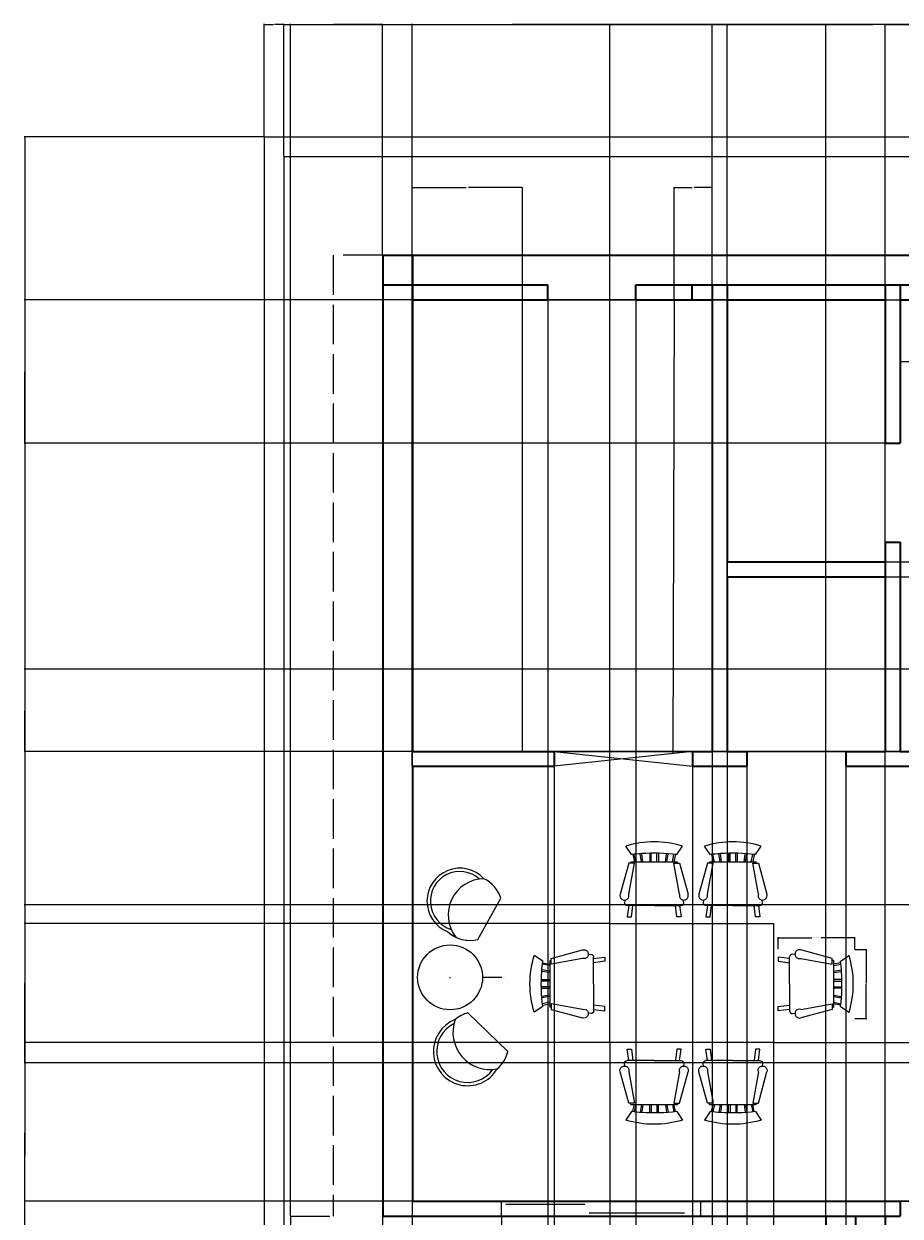
# Model space of a CAD drawing. Units: inches. Extents: x -47 to 496, y -43 to 706.
# Tile 5 of 6: x -47 to 218, y 344 to 706. Entities that reach past the tile are written whole.
import ezdxf

# ---------------------------------------------------------------- set-up
doc = ezdxf.new("R2010")
doc.units = ezdxf.units.IN
doc.linetypes.add('ACAD_ISO02W100', pattern=[15, 12, -3])
for name, color, linetype, lineweight in [('A-ANNO-DIMS', 2, 'Continuous', 18), ('A-FLOR-CASE', 3, 'Continuous', 18), ('A-ROOF-OVHD', 8, 'ACAD_ISO02W100', 18), ('C-PROP', 7, 'Continuous', 25), ('DOOR', 4, 'Continuous', 25), ('FURNITURE', 3, 'Continuous', 18), ('WALL', 7, 'Continuous', 35), ('WINDOW', 1, 'Continuous', 18)]:
    doc.layers.add(name, color=color, linetype=linetype, lineweight=lineweight)
doc.styles.get("Standard").update_dxf_attribs({"font": 'arial.ttf'})
doc.dimstyles.get("Standard").update_dxf_attribs({"dimtxt": 0.18, "dimasz": 0.18, "dimexe": 0.18, "dimexo": 0.0625, "dimgap": 0.09, "dimtad": 0, "dimtih": 1, "dimtoh": 1, "dimdec": 4, "dimzin": 0, "dimdsep": 46, "dimtxsty": 'Standard', "dimcen": 0.09, "dimadec": 0, "dimazin": 0, "dimtfac": 1, "dimtdec": 4, "dimtofl": 0, "dimtmove": 0, "dimatfit": 3, "dimfxl": 1, "dimtolj": 1, "dimtzin": 0, "dimarcsym": 0})

# ---------------------------------------------------------------- blocks, each defined once
blk = doc.blocks.new('Chair - Rocking')
for p, q in [((-8, -4.5), (-10, -1.5)), ((-4.5, -7), (-4.96674, -4.19951)), ((-4, -7), (-4.40532, -4.16272)), ((-1.5, -4.05012), (-1.5, -7)), ((-1, -7), (-1, -4.05012)), ((1, -7), (1, -4.04655)), ((1.5, -4.05012), (1.5, -7)), ((4, -7), (4.40187, -4.18694)), ((4.5, -7), (4.96761, -4.19437)), ((8, -4.5), (10, -1.5)), ((-9, -7.5), (-12, -18.49999)), ((-7, -7.5), (-9, -7.5)), ((-9, -18.49999), (-7, -7.5)), ((-8.23428, -6.99939), (-8.3093, -7.47958)), ((-8.23041, -7), (8.23915, -7)), ((-7.5, -4.5), (-7, -7)), ((-6.5, -7), (-7.02225, -4.43)), ((6.5, -7), (7, -4.4057)), ((7.5, -4.5), (7, -7)), ((7, -7.5), (9, -7.5)), ((9, -18.49999), (7, -7.5)), ((8.31071, -7.48854), (8.23449, -7.00073)), ((9, -7.5), (12, -18.49999)), ((-10.36644, -20.64523), (-10.5, -21.49999)), ((10.5, -21.49999), (10.3575, -20.58798)), ((-9, -22.49999), (-9.5, -26.49999)), ((0, -22.49999), (-9.5, -22.49999)), ((-8, -26.49999), (-7.5, -22.49999)), ((0, -22.49999), (9.5, -22.49999)), ((8, -26.49999), (7.5, -22.49999)), ((9, -22.49999), (9.5, -26.49999)), ((-9.5, -26.49999), (-8, -26.49999)), ((9.5, -26.49999), (8, -26.49999))]:
    blk.add_line(p, q)
for centre, radius, start, end in [((0, -34.08333), 34.08333, 72.93847, 107.0615), ((0, -68.25004), 64.25, 93.92211, 97.15267), ((0, -68.25004), 64.25, 82.84733, 93.92211), ((-10.5, -18.99999), 1.58114, 161.5651, 18.43495), ((10.5, -18.99999), 1.58114, 161.5651, 18.43495), ((-9.5, -21.49999), 1, 180, 270), ((9.5, -21.49999), 1, 270, 0)]:
    blk.add_arc(centre, radius, start, end)
blk = doc.blocks.new('*D8')
at = {"layer": 'A-ANNO-DIMS', "color": 0, "lineweight": -2, "transparency": 16777216}
for p, q in [((181.49, 424.98), (181.49, 428.58)), ((181.67, 428.4), (191.66, 428.4)), ((204.49, 428.4), (194.51, 428.4)), ((204.67, 424.98), (204.67, 428.58))]:
    blk.add_line(p, q, dxfattribs=at)
at = {"layer": 'A-ANNO-DIMS', "color": 0, "transparency": 16777216}
for points in [[(181.67, 428.43), (181.67, 428.37), (181.49, 428.4)], [(204.49, 428.43), (204.49, 428.37), (204.67, 428.4)]]:
    blk.add_solid(points, dxfattribs=at)
at = {"layer": 'Defpoints', "color": 0, "transparency": 16777216}
for p in [(204.67, 428.4), (181.49, 424.92), (204.67, 424.92)]:
    blk.add_point(p, dxfattribs=at)
at = {"layer": 'A-ANNO-DIMS', "color": 0, "transparency": 16777216, "insert": (193.08, 428.4), "char_height": 0.18, "attachment_point": 5}
blk.add_mtext('\\A1;DINING CHAIR 23 TYP.', dxfattribs=at)
blk = doc.blocks.new('*D9')
at = {"layer": 'A-ANNO-DIMS', "color": 0, "lineweight": -2, "transparency": 16777216}
for p, q in [((204.73, 424.92), (208.33, 424.92)), ((208.15, 424.74), (208.15, 414.61)), ((208.15, 404.12), (208.15, 414.25)), ((204.73, 403.94), (208.33, 403.94))]:
    blk.add_line(p, q, dxfattribs=at)
at = {"layer": 'A-ANNO-DIMS', "color": 0, "transparency": 16777216}
for points in [[(208.12, 424.74), (208.18, 424.74), (208.15, 424.92)], [(208.12, 404.12), (208.18, 404.12), (208.15, 403.94)]]:
    blk.add_solid(points, dxfattribs=at)
at = {"layer": 'Defpoints', "color": 0, "transparency": 16777216}
for p in [(204.67, 424.92), (204.67, 403.94), (208.15, 403.94)]:
    blk.add_point(p, dxfattribs=at)
at = {"layer": 'A-ANNO-DIMS', "color": 0, "transparency": 16777216, "insert": (208.15, 414.43), "char_height": 0.18, "attachment_point": 5}
blk.add_mtext('\\A1;21 TYP.', dxfattribs=at)
blk = doc.blocks.new('*D13')
at = {"layer": 'A-ANNO-DIMS', "color": 0, "lineweight": -2, "transparency": 16777216}
for p, q in [((25.39, 671.47), (-47.29, 671.47)), ((-47.11, 671.29), (-47.11, 362.4)), ((-47.11, 53.15), (-47.11, 362.04)), ((25.39, 52.97), (-47.29, 52.97))]:
    blk.add_line(p, q, dxfattribs=at)
at = {"layer": 'A-ANNO-DIMS', "color": 0, "transparency": 16777216}
for points in [[(-47.14, 671.29), (-47.08, 671.29), (-47.11, 671.47)], [(-47.14, 53.15), (-47.08, 53.15), (-47.11, 52.97)]]:
    blk.add_solid(points, dxfattribs=at)
at = {"layer": 'Defpoints', "color": 0, "transparency": 16777216}
for p in [(-47.11, 671.47), (25.45, 671.47), (25.45, 52.97)]:
    blk.add_point(p, dxfattribs=at)
at = {"layer": 'A-ANNO-DIMS', "color": 0, "transparency": 16777216, "insert": (-47.11, 362.22), "char_height": 0.18, "attachment_point": 5}
blk.add_mtext('\\A1;618.5', dxfattribs=at)
blk = doc.blocks.new('*D14')
at = {"layer": 'A-ANNO-DIMS', "color": 0, "lineweight": -2, "transparency": 16777216}
for p, q in [((25.45, 671.53), (25.45, 705.7)), ((25.63, 705.52), (28.31, 705.52)), ((31.27, 705.52), (28.6, 705.52)), ((31.45, 665.53), (31.45, 705.7))]:
    blk.add_line(p, q, dxfattribs=at)
at = {"layer": 'A-ANNO-DIMS', "color": 0, "transparency": 16777216}
for points in [[(25.63, 705.55), (25.63, 705.49), (25.45, 705.52)], [(31.27, 705.55), (31.27, 705.49), (31.45, 705.52)]]:
    blk.add_solid(points, dxfattribs=at)
at = {"layer": 'Defpoints', "color": 0, "transparency": 16777216}
for p in [(31.45, 705.52), (25.45, 671.47), (31.45, 665.47)]:
    blk.add_point(p, dxfattribs=at)
at = {"layer": 'A-ANNO-DIMS', "color": 0, "transparency": 16777216, "insert": (28.45, 705.52), "char_height": 0.18, "attachment_point": 5}
blk.add_mtext('\\A1;6', dxfattribs=at)
blk = doc.blocks.new('*D15')
at = {"layer": 'A-ANNO-DIMS', "color": 0, "lineweight": -2, "transparency": 16777216}
for p, q in [((31.45, 665.53), (31.45, 705.7)), ((31.63, 705.52), (46.24, 705.52)), ((61.27, 705.52), (46.67, 705.52)), ((61.45, 635.53), (61.45, 705.7))]:
    blk.add_line(p, q, dxfattribs=at)
at = {"layer": 'A-ANNO-DIMS', "color": 0, "transparency": 16777216}
for points in [[(31.63, 705.55), (31.63, 705.49), (31.45, 705.52)], [(61.27, 705.55), (61.27, 705.49), (61.45, 705.52)]]:
    blk.add_solid(points, dxfattribs=at)
at = {"layer": 'Defpoints', "color": 0, "transparency": 16777216}
for p in [(61.45, 705.52), (31.45, 665.47), (61.45, 635.47)]:
    blk.add_point(p, dxfattribs=at)
at = {"layer": 'A-ANNO-DIMS', "color": 0, "transparency": 16777216, "insert": (46.45, 705.52), "char_height": 0.18, "attachment_point": 5}
blk.add_mtext('\\A1;30', dxfattribs=at)
blk = doc.blocks.new('*D26')
at = {"layer": 'A-ANNO-DIMS', "color": 0, "lineweight": -2, "transparency": 16777216}
for p, q in [((213.95, 131.03), (213.95, 705.7)), ((214.13, 705.52), (221.46, 705.52)), ((229.7, 705.52), (222.37, 705.52)), ((229.88, 163.9), (229.88, 705.7))]:
    blk.add_line(p, q, dxfattribs=at)
at = {"layer": 'A-ANNO-DIMS', "color": 0, "transparency": 16777216}
for points in [[(214.13, 705.55), (214.13, 705.49), (213.95, 705.52)], [(229.7, 705.55), (229.7, 705.49), (229.88, 705.52)]]:
    blk.add_solid(points, dxfattribs=at)
at = {"layer": 'Defpoints', "color": 0, "transparency": 16777216}
for p in [(229.88, 705.52), (229.88, 163.83), (213.95, 130.97)]:
    blk.add_point(p, dxfattribs=at)
at = {"layer": 'A-ANNO-DIMS', "color": 0, "transparency": 16777216, "insert": (221.92, 705.52), "char_height": 0.18, "attachment_point": 5}
blk.add_mtext('\\A1;15.924', dxfattribs=at)
blk = doc.blocks.new('*D32')
at = {"layer": 'A-ANNO-DIMS', "color": 0, "lineweight": -2, "transparency": 16777216}
for p, q in [((61.45, 635.53), (61.45, 705.7)), ((61.63, 705.52), (210.16, 705.52)), ((359.27, 705.52), (210.75, 705.52)), ((359.45, 635.53), (359.45, 705.7))]:
    blk.add_line(p, q, dxfattribs=at)
at = {"layer": 'A-ANNO-DIMS', "color": 0, "transparency": 16777216}
for points in [[(61.63, 705.55), (61.63, 705.49), (61.45, 705.52)], [(359.27, 705.55), (359.27, 705.49), (359.45, 705.52)]]:
    blk.add_solid(points, dxfattribs=at)
at = {"layer": 'Defpoints', "color": 0, "transparency": 16777216}
for p in [(359.45, 705.52), (61.45, 635.47), (359.45, 635.47)]:
    blk.add_point(p, dxfattribs=at)
at = {"layer": 'A-ANNO-DIMS', "color": 0, "transparency": 16777216, "insert": (210.45, 705.52), "char_height": 0.18, "attachment_point": 5}
blk.add_mtext('\\A1;298', dxfattribs=at)
blk = doc.blocks.new('*D33')
at = {"layer": 'A-ANNO-DIMS', "color": 0, "lineweight": -2, "transparency": 16777216}
for p, q in [((70.45, 485.03), (70.45, 705.7)), ((70.63, 705.52), (115.75, 705.52)), ((161.27, 705.52), (116.16, 705.52)), ((161.45, 485.03), (161.45, 705.7))]:
    blk.add_line(p, q, dxfattribs=at)
at = {"layer": 'A-ANNO-DIMS', "color": 0, "transparency": 16777216}
for points in [[(70.63, 705.55), (70.63, 705.49), (70.45, 705.52)], [(161.27, 705.55), (161.27, 705.49), (161.45, 705.52)]]:
    blk.add_solid(points, dxfattribs=at)
at = {"layer": 'Defpoints', "color": 0, "transparency": 16777216}
for p in [(161.45, 705.52), (70.45, 484.97), (161.45, 484.97)]:
    blk.add_point(p, dxfattribs=at)
at = {"layer": 'A-ANNO-DIMS', "color": 0, "transparency": 16777216, "insert": (115.95, 705.52), "char_height": 0.18, "attachment_point": 5}
blk.add_mtext('\\A1;91', dxfattribs=at)
blk = doc.blocks.new('*D34')
at = {"layer": 'A-ANNO-DIMS', "color": 0, "lineweight": -2, "transparency": 16777216}
for p, q in [((165.95, 485.03), (165.95, 705.7)), ((166.13, 705.52), (189.73, 705.52)), ((213.77, 705.52), (190.18, 705.52)), ((213.95, 485.03), (213.95, 705.7))]:
    blk.add_line(p, q, dxfattribs=at)
at = {"layer": 'A-ANNO-DIMS', "color": 0, "transparency": 16777216}
for points in [[(166.13, 705.55), (166.13, 705.49), (165.95, 705.52)], [(213.77, 705.55), (213.77, 705.49), (213.95, 705.52)]]:
    blk.add_solid(points, dxfattribs=at)
at = {"layer": 'Defpoints', "color": 0, "transparency": 16777216}
for p in [(213.95, 705.52), (165.95, 484.97), (213.95, 484.97)]:
    blk.add_point(p, dxfattribs=at)
at = {"layer": 'A-ANNO-DIMS', "color": 0, "transparency": 16777216, "insert": (189.95, 705.52), "char_height": 0.18, "attachment_point": 5}
blk.add_mtext('\\A1;48', dxfattribs=at)
blk = doc.blocks.new('*D36')
at = {"layer": 'A-ANNO-DIMS', "color": 0, "lineweight": -2, "transparency": 16777216}
for p, q in [((70.52, 621.97), (496.14, 621.97)), ((495.96, 621.79), (495.96, 553.65)), ((495.96, 485.15), (495.96, 553.29)), ((70.52, 484.97), (496.14, 484.97))]:
    blk.add_line(p, q, dxfattribs=at)
at = {"layer": 'A-ANNO-DIMS', "color": 0, "transparency": 16777216}
for points in [[(495.93, 621.79), (495.99, 621.79), (495.96, 621.97)], [(495.93, 485.15), (495.99, 485.15), (495.96, 484.97)]]:
    blk.add_solid(points, dxfattribs=at)
at = {"layer": 'Defpoints', "color": 0, "transparency": 16777216}
for p in [(70.45, 621.97), (495.96, 621.97), (70.45, 484.97)]:
    blk.add_point(p, dxfattribs=at)
at = {"layer": 'A-ANNO-DIMS', "color": 0, "transparency": 16777216, "insert": (495.96, 553.47), "char_height": 0.18, "attachment_point": 5}
blk.add_mtext('\\A1;137', dxfattribs=at)
blk = doc.blocks.new('*D37')
at = {"layer": 'A-ANNO-DIMS', "color": 0, "lineweight": -2, "transparency": 16777216}
for p, q in [((166.02, 621.97), (496.14, 621.97)), ((495.96, 621.79), (495.96, 582.4)), ((495.96, 542.65), (495.96, 582.04)), ((166.02, 542.47), (496.14, 542.47))]:
    blk.add_line(p, q, dxfattribs=at)
at = {"layer": 'A-ANNO-DIMS', "color": 0, "transparency": 16777216}
for points in [[(495.93, 621.79), (495.99, 621.79), (495.96, 621.97)], [(495.93, 542.65), (495.99, 542.65), (495.96, 542.47)]]:
    blk.add_solid(points, dxfattribs=at)
at = {"layer": 'Defpoints', "color": 0, "transparency": 16777216}
for p in [(165.95, 621.97), (495.96, 621.97), (165.95, 542.47)]:
    blk.add_point(p, dxfattribs=at)
at = {"layer": 'A-ANNO-DIMS', "color": 0, "transparency": 16777216, "insert": (495.96, 582.22), "char_height": 0.18, "attachment_point": 5}
blk.add_mtext('\\A1;79.5', dxfattribs=at)
blk = doc.blocks.new('*D38')
at = {"layer": 'A-ANNO-DIMS', "color": 0, "lineweight": -2, "transparency": 16777216}
for p, q in [((166.02, 537.97), (496.14, 537.97)), ((495.96, 537.79), (495.96, 511.65)), ((495.96, 485.15), (495.96, 511.29)), ((166.02, 484.97), (496.14, 484.97))]:
    blk.add_line(p, q, dxfattribs=at)
at = {"layer": 'A-ANNO-DIMS', "color": 0, "transparency": 16777216}
for points in [[(495.93, 537.79), (495.99, 537.79), (495.96, 537.97)], [(495.93, 485.15), (495.99, 485.15), (495.96, 484.97)]]:
    blk.add_solid(points, dxfattribs=at)
at = {"layer": 'Defpoints', "color": 0, "transparency": 16777216}
for p in [(165.95, 537.97), (495.96, 537.97), (165.95, 484.97)]:
    blk.add_point(p, dxfattribs=at)
at = {"layer": 'A-ANNO-DIMS', "color": 0, "transparency": 16777216, "insert": (495.96, 511.47), "char_height": 0.18, "attachment_point": 5}
blk.add_mtext('\\A1;53', dxfattribs=at)
blk = doc.blocks.new('*D40')
at = {"layer": 'A-ANNO-DIMS', "color": 0, "lineweight": -2, "transparency": 16777216}
for p, q in [((213.89, 621.97), (-47.29, 621.97)), ((-47.11, 621.79), (-47.11, 600.4)), ((-47.11, 578.65), (-47.11, 600.04)), ((213.89, 578.47), (-47.29, 578.47))]:
    blk.add_line(p, q, dxfattribs=at)
at = {"layer": 'A-ANNO-DIMS', "color": 0, "transparency": 16777216}
for points in [[(-47.14, 621.79), (-47.08, 621.79), (-47.11, 621.97)], [(-47.14, 578.65), (-47.08, 578.65), (-47.11, 578.47)]]:
    blk.add_solid(points, dxfattribs=at)
at = {"layer": 'Defpoints', "color": 0, "transparency": 16777216}
for p in [(-47.11, 621.97), (213.95, 621.97), (213.95, 578.47)]:
    blk.add_point(p, dxfattribs=at)
at = {"layer": 'A-ANNO-DIMS', "color": 0, "transparency": 16777216, "insert": (-47.11, 600.22), "char_height": 0.18, "attachment_point": 5}
blk.add_mtext('\\A1;43.5', dxfattribs=at)
blk = doc.blocks.new('*D41')
at = {"layer": 'A-ANNO-DIMS', "color": 0, "lineweight": -2, "transparency": 16777216}
for p, q in [((111.58, 621.91), (111.58, -42.84)), ((138.26, 621.91), (138.26, -42.84)), ((111.76, -42.66), (124.45, -42.66)), ((138.08, -42.66), (125.38, -42.66))]:
    blk.add_line(p, q, dxfattribs=at)
at = {"layer": 'A-ANNO-DIMS', "color": 0, "transparency": 16777216}
for points in [[(111.76, -42.63), (111.76, -42.69), (111.58, -42.66)], [(138.08, -42.63), (138.08, -42.69), (138.26, -42.66)]]:
    blk.add_solid(points, dxfattribs=at)
at = {"layer": 'Defpoints', "color": 0, "transparency": 16777216}
for p in [(111.58, 621.97), (138.26, 621.97), (138.26, -42.66)]:
    blk.add_point(p, dxfattribs=at)
at = {"layer": 'A-ANNO-DIMS', "color": 0, "transparency": 16777216, "insert": (124.92, -42.66), "char_height": 0.18, "attachment_point": 5}
blk.add_mtext('\\A1;26.675', dxfattribs=at)
blk = doc.blocks.new('*D42')
at = {"layer": 'A-ANNO-DIMS', "color": 0, "lineweight": -2, "transparency": 16777216}
for p, q in [((70.45, 621.91), (70.45, -42.84)), ((111.58, 621.91), (111.58, -42.84)), ((70.63, -42.66), (90.55, -42.66)), ((111.4, -42.66), (91.48, -42.66))]:
    blk.add_line(p, q, dxfattribs=at)
at = {"layer": 'A-ANNO-DIMS', "color": 0, "transparency": 16777216}
for points in [[(70.63, -42.63), (70.63, -42.69), (70.45, -42.66)], [(111.4, -42.63), (111.4, -42.69), (111.58, -42.66)]]:
    blk.add_solid(points, dxfattribs=at)
at = {"layer": 'Defpoints', "color": 0, "transparency": 16777216}
for p in [(70.45, 621.97), (111.58, 621.97), (111.58, -42.66)]:
    blk.add_point(p, dxfattribs=at)
at = {"layer": 'A-ANNO-DIMS', "color": 0, "transparency": 16777216, "insert": (91.02, -42.66), "char_height": 0.18, "attachment_point": 5}
blk.add_mtext('\\A1;41.125', dxfattribs=at)
blk = doc.blocks.new('*D43')
at = {"layer": 'A-ANNO-DIMS', "color": 0, "lineweight": -2, "transparency": 16777216}
for p, q in [((70.45, 622.03), (70.45, 656.2)), ((70.63, 656.02), (86.83, 656.02)), ((103.67, 656.02), (87.48, 656.02)), ((103.85, 622.03), (103.85, 656.2))]:
    blk.add_line(p, q, dxfattribs=at)
at = {"layer": 'A-ANNO-DIMS', "color": 0, "transparency": 16777216}
for points in [[(70.63, 656.05), (70.63, 655.99), (70.45, 656.02)], [(103.67, 656.05), (103.67, 655.99), (103.85, 656.02)]]:
    blk.add_solid(points, dxfattribs=at)
at = {"layer": 'Defpoints', "color": 0, "transparency": 16777216}
for p in [(103.85, 656.02), (70.45, 621.97), (103.85, 621.97)]:
    blk.add_point(p, dxfattribs=at)
at = {"layer": 'A-ANNO-DIMS', "color": 0, "transparency": 16777216, "insert": (87.15, 656.02), "char_height": 0.18, "attachment_point": 5}
blk.add_mtext('\\A1;33.4', dxfattribs=at)
blk = doc.blocks.new('*D44')
at = {"layer": 'A-ANNO-DIMS', "color": 0, "lineweight": -2, "transparency": 16777216}
for p, q in [((149.85, 622.03), (149.85, 656.2)), ((150.03, 656.02), (155.34, 656.02)), ((161.27, 656.02), (155.97, 656.02)), ((161.45, 622.03), (161.45, 656.2))]:
    blk.add_line(p, q, dxfattribs=at)
at = {"layer": 'A-ANNO-DIMS', "color": 0, "transparency": 16777216}
for points in [[(150.03, 656.05), (150.03, 655.99), (149.85, 656.02)], [(161.27, 656.05), (161.27, 655.99), (161.45, 656.02)]]:
    blk.add_solid(points, dxfattribs=at)
at = {"layer": 'Defpoints', "color": 0, "transparency": 16777216}
for p in [(161.45, 656.02), (149.85, 621.97), (161.45, 621.97)]:
    blk.add_point(p, dxfattribs=at)
at = {"layer": 'A-ANNO-DIMS', "color": 0, "transparency": 16777216, "insert": (155.65, 656.02), "char_height": 0.18, "attachment_point": 5}
blk.add_mtext('\\A1;11.6', dxfattribs=at)
blk = doc.blocks.new('*D45')
at = {"layer": 'A-ANNO-DIMS', "color": 0, "lineweight": -2, "transparency": 16777216}
for p, q in [((113.45, 480.41), (113.45, -42.84)), ((155.45, 480.41), (155.45, -42.84)), ((113.63, -42.66), (134.23, -42.66)), ((155.27, -42.66), (134.68, -42.66))]:
    blk.add_line(p, q, dxfattribs=at)
at = {"layer": 'A-ANNO-DIMS', "color": 0, "transparency": 16777216}
for points in [[(113.63, -42.63), (113.63, -42.69), (113.45, -42.66)], [(155.27, -42.63), (155.27, -42.69), (155.45, -42.66)]]:
    blk.add_solid(points, dxfattribs=at)
at = {"layer": 'Defpoints', "color": 0, "transparency": 16777216}
for p in [(113.45, 480.47), (155.45, 480.47), (155.45, -42.66)]:
    blk.add_point(p, dxfattribs=at)
at = {"layer": 'A-ANNO-DIMS', "color": 0, "transparency": 16777216, "insert": (134.45, -42.66), "char_height": 0.18, "attachment_point": 5}
blk.add_mtext('\\A1;42', dxfattribs=at)
blk = doc.blocks.new('*D46')
at = {"layer": 'A-ANNO-DIMS', "color": 0, "lineweight": -2, "transparency": 16777216}
for p, q in [((70.45, 480.41), (70.45, -42.84)), ((113.45, 480.41), (113.45, -42.84)), ((70.63, -42.66), (91.73, -42.66)), ((113.27, -42.66), (92.18, -42.66))]:
    blk.add_line(p, q, dxfattribs=at)
at = {"layer": 'A-ANNO-DIMS', "color": 0, "transparency": 16777216}
for points in [[(70.63, -42.63), (70.63, -42.69), (70.45, -42.66)], [(113.27, -42.63), (113.27, -42.69), (113.45, -42.66)]]:
    blk.add_solid(points, dxfattribs=at)
at = {"layer": 'Defpoints', "color": 0, "transparency": 16777216}
for p in [(70.45, 480.47), (113.45, 480.47), (113.45, -42.66)]:
    blk.add_point(p, dxfattribs=at)
at = {"layer": 'A-ANNO-DIMS', "color": 0, "transparency": 16777216, "insert": (91.95, -42.66), "char_height": 0.18, "attachment_point": 5}
blk.add_mtext('\\A1;43', dxfattribs=at)
blk = doc.blocks.new('*D47')
at = {"layer": 'A-ANNO-DIMS', "color": 0, "lineweight": -2, "transparency": 16777216}
for p, q in [((171.95, 480.41), (171.95, -42.84)), ((201.95, 480.41), (201.95, -42.84)), ((172.13, -42.66), (186.74, -42.66)), ((201.77, -42.66), (187.17, -42.66))]:
    blk.add_line(p, q, dxfattribs=at)
at = {"layer": 'A-ANNO-DIMS', "color": 0, "transparency": 16777216}
for points in [[(172.13, -42.63), (172.13, -42.69), (171.95, -42.66)], [(201.77, -42.63), (201.77, -42.69), (201.95, -42.66)]]:
    blk.add_solid(points, dxfattribs=at)
at = {"layer": 'Defpoints', "color": 0, "transparency": 16777216}
for p in [(171.95, 480.47), (201.95, 480.47), (201.95, -42.66)]:
    blk.add_point(p, dxfattribs=at)
at = {"layer": 'A-ANNO-DIMS', "color": 0, "transparency": 16777216, "insert": (186.95, -42.66), "char_height": 0.18, "attachment_point": 5}
blk.add_mtext('\\A1;30', dxfattribs=at)
blk = doc.blocks.new('*D49')
at = {"layer": 'A-ANNO-DIMS', "color": 0, "lineweight": -2, "transparency": 16777216}
for p, q in [((61.45, 635.41), (61.45, -42.84)), ((70.45, 635.41), (70.45, -42.84)), ((61.63, -42.66), (65.81, -42.66)), ((70.27, -42.66), (66.1, -42.66))]:
    blk.add_line(p, q, dxfattribs=at)
at = {"layer": 'A-ANNO-DIMS', "color": 0, "transparency": 16777216}
for points in [[(61.63, -42.63), (61.63, -42.69), (61.45, -42.66)], [(70.27, -42.63), (70.27, -42.69), (70.45, -42.66)]]:
    blk.add_solid(points, dxfattribs=at)
at = {"layer": 'Defpoints', "color": 0, "transparency": 16777216}
for p in [(61.45, 635.47), (70.45, 635.47), (70.45, -42.66)]:
    blk.add_point(p, dxfattribs=at)
at = {"layer": 'A-ANNO-DIMS', "color": 0, "transparency": 16777216, "insert": (65.95, -42.66), "char_height": 0.18, "attachment_point": 5}
blk.add_mtext('\\A1;9', dxfattribs=at)
blk = doc.blocks.new('*D50')
at = {"layer": 'A-ANNO-DIMS', "color": 0, "lineweight": -2, "transparency": 16777216}
for p, q in [((161.45, 621.91), (161.45, -42.84)), ((165.95, 621.91), (165.95, -42.84)), ((161.63, -42.66), (163.45, -42.66)), ((165.77, -42.66), (163.96, -42.66))]:
    blk.add_line(p, q, dxfattribs=at)
at = {"layer": 'A-ANNO-DIMS', "color": 0, "transparency": 16777216}
for points in [[(161.63, -42.63), (161.63, -42.69), (161.45, -42.66)], [(165.77, -42.63), (165.77, -42.69), (165.95, -42.66)]]:
    blk.add_solid(points, dxfattribs=at)
at = {"layer": 'Defpoints', "color": 0, "transparency": 16777216}
for p in [(161.45, 621.97), (165.95, 621.97), (165.95, -42.66)]:
    blk.add_point(p, dxfattribs=at)
at = {"layer": 'A-ANNO-DIMS', "color": 0, "transparency": 16777216, "insert": (163.7, -42.66), "char_height": 0.18, "attachment_point": 5}
blk.add_mtext('\\A1;4.5', dxfattribs=at)
blk = doc.blocks.new('*D53')
at = {"layer": 'A-ANNO-DIMS', "color": 0, "lineweight": -2, "transparency": 16777216}
for p, q in [((266.39, 509.97), (-47.29, 509.97)), ((-47.11, 509.79), (-47.11, 497.65)), ((-47.11, 485.15), (-47.11, 497.29)), ((266.39, 484.97), (-47.29, 484.97))]:
    blk.add_line(p, q, dxfattribs=at)
at = {"layer": 'A-ANNO-DIMS', "color": 0, "transparency": 16777216}
for points in [[(-47.14, 509.79), (-47.08, 509.79), (-47.11, 509.97)], [(-47.14, 485.15), (-47.08, 485.15), (-47.11, 484.97)]]:
    blk.add_solid(points, dxfattribs=at)
at = {"layer": 'Defpoints', "color": 0, "transparency": 16777216}
for p in [(-47.11, 509.97), (266.45, 509.97), (266.45, 484.97)]:
    blk.add_point(p, dxfattribs=at)
at = {"layer": 'A-ANNO-DIMS', "color": 0, "transparency": 16777216, "insert": (-47.11, 497.47), "char_height": 0.18, "attachment_point": 5}
blk.add_mtext('\\A1;25', dxfattribs=at)
blk = doc.blocks.new('*D57')
at = {"layer": 'A-ANNO-DIMS', "color": 0, "lineweight": -2, "transparency": 16777216}
for p, q in [((273.42, 438.47), (-47.29, 438.47)), ((-47.11, 438.29), (-47.11, 414.65)), ((-47.11, 390.65), (-47.11, 414.29)), ((273.42, 390.47), (-47.29, 390.47))]:
    blk.add_line(p, q, dxfattribs=at)
at = {"layer": 'A-ANNO-DIMS', "color": 0, "transparency": 16777216}
for points in [[(-47.14, 438.29), (-47.08, 438.29), (-47.11, 438.47)], [(-47.14, 390.65), (-47.08, 390.65), (-47.11, 390.47)]]:
    blk.add_solid(points, dxfattribs=at)
at = {"layer": 'Defpoints', "color": 0, "transparency": 16777216}
for p in [(-47.11, 438.47), (273.48, 438.47), (273.48, 390.47)]:
    blk.add_point(p, dxfattribs=at)
at = {"layer": 'A-ANNO-DIMS', "color": 0, "transparency": 16777216, "insert": (-47.11, 414.47), "char_height": 0.18, "attachment_point": 5}
blk.add_mtext('\\A1;48', dxfattribs=at)
blk = doc.blocks.new('*D58')
at = {"layer": 'A-ANNO-DIMS', "color": 0, "lineweight": -2, "transparency": 16777216}
for p, q in [((273.42, 390.47), (-47.29, 390.47)), ((-47.11, 390.29), (-47.11, 369.65)), ((-47.11, 348.65), (-47.11, 369.29)), ((273.42, 348.47), (-47.29, 348.47))]:
    blk.add_line(p, q, dxfattribs=at)
at = {"layer": 'A-ANNO-DIMS', "color": 0, "transparency": 16777216}
for points in [[(-47.14, 390.29), (-47.08, 390.29), (-47.11, 390.47)], [(-47.14, 348.65), (-47.08, 348.65), (-47.11, 348.47)]]:
    blk.add_solid(points, dxfattribs=at)
at = {"layer": 'Defpoints', "color": 0, "transparency": 16777216}
for p in [(-47.11, 390.47), (273.48, 390.47), (273.48, 348.47)]:
    blk.add_point(p, dxfattribs=at)
at = {"layer": 'A-ANNO-DIMS', "color": 0, "transparency": 16777216, "insert": (-47.11, 369.47), "char_height": 0.18, "attachment_point": 5}
blk.add_mtext('\\A1;42', dxfattribs=at)
blk = doc.blocks.new('*D62')
at = {"layer": 'A-ANNO-DIMS', "color": 0, "lineweight": -2, "transparency": 16777216}
for p, q in [((70.45, 348.41), (70.45, -42.84)), ((97.54, 343.91), (97.54, -42.84)), ((70.63, -42.66), (83.6, -42.66)), ((97.36, -42.66), (84.39, -42.66))]:
    blk.add_line(p, q, dxfattribs=at)
at = {"layer": 'A-ANNO-DIMS', "color": 0, "transparency": 16777216}
for points in [[(70.63, -42.63), (70.63, -42.69), (70.45, -42.66)], [(97.36, -42.63), (97.36, -42.69), (97.54, -42.66)]]:
    blk.add_solid(points, dxfattribs=at)
at = {"layer": 'Defpoints', "color": 0, "transparency": 16777216}
for p in [(70.45, 348.47), (97.54, 343.97), (97.54, -42.66)]:
    blk.add_point(p, dxfattribs=at)
at = {"layer": 'A-ANNO-DIMS', "color": 0, "transparency": 16777216, "insert": (84, -42.66), "char_height": 0.18, "attachment_point": 5}
blk.add_mtext('\\A1;27.09', dxfattribs=at)
blk = doc.blocks.new('*D66')
at = {"layer": 'A-ANNO-DIMS', "color": 0, "lineweight": -2, "transparency": 16777216}
for p, q in [((130.34, 396.56), (130.34, -42.84)), ((180.05, 396.56), (180.05, -42.84)), ((130.52, -42.66), (154.82, -42.66)), ((179.87, -42.66), (155.58, -42.66))]:
    blk.add_line(p, q, dxfattribs=at)
at = {"layer": 'A-ANNO-DIMS', "color": 0, "transparency": 16777216}
for points in [[(130.52, -42.63), (130.52, -42.69), (130.34, -42.66)], [(179.87, -42.63), (179.87, -42.69), (180.05, -42.66)]]:
    blk.add_solid(points, dxfattribs=at)
at = {"layer": 'Defpoints', "color": 0, "transparency": 16777216}
for p in [(130.34, 396.63), (180.05, 396.63), (180.05, -42.66)]:
    blk.add_point(p, dxfattribs=at)
at = {"layer": 'A-ANNO-DIMS', "color": 0, "transparency": 16777216, "insert": (155.2, -42.66), "char_height": 0.18, "attachment_point": 5}
blk.add_mtext('\\A1;49.71', dxfattribs=at)
blk = doc.blocks.new('*D67')
at = {"layer": 'A-ANNO-DIMS', "color": 0, "lineweight": -2, "transparency": 16777216}
for p, q in [((130.28, 432.74), (-47.29, 432.74)), ((-47.11, 432.56), (-47.11, 414.86)), ((-47.11, 396.81), (-47.11, 414.5)), ((130.28, 396.63), (-47.29, 396.63))]:
    blk.add_line(p, q, dxfattribs=at)
at = {"layer": 'A-ANNO-DIMS', "color": 0, "transparency": 16777216}
for points in [[(-47.14, 432.56), (-47.08, 432.56), (-47.11, 432.74)], [(-47.14, 396.81), (-47.08, 396.81), (-47.11, 396.63)]]:
    blk.add_solid(points, dxfattribs=at)
at = {"layer": 'Defpoints', "color": 0, "transparency": 16777216}
for p in [(-47.11, 432.74), (130.34, 432.74), (130.34, 396.63)]:
    blk.add_point(p, dxfattribs=at)
at = {"layer": 'A-ANNO-DIMS', "color": 0, "transparency": 16777216, "insert": (-47.11, 414.68), "char_height": 0.18, "attachment_point": 5}
blk.add_mtext('\\A1;36.11', dxfattribs=at)
blk = doc.blocks.new('*D68')
at = {"layer": 'A-ANNO-DIMS', "color": 0, "lineweight": -2, "transparency": 16777216}
for p, q in [((70.45, 480.53), (70.45, 705.7)), ((70.63, 705.52), (100, 705.52)), ((130.16, 705.52), (100.79, 705.52)), ((130.34, 432.8), (130.34, 705.7))]:
    blk.add_line(p, q, dxfattribs=at)
at = {"layer": 'A-ANNO-DIMS', "color": 0, "transparency": 16777216}
for points in [[(70.63, 705.55), (70.63, 705.49), (70.45, 705.52)], [(130.16, 705.55), (130.16, 705.49), (130.34, 705.52)]]:
    blk.add_solid(points, dxfattribs=at)
at = {"layer": 'Defpoints', "color": 0, "transparency": 16777216}
for p in [(130.34, 705.52), (70.45, 480.47), (130.34, 432.74)]:
    blk.add_point(p, dxfattribs=at)
at = {"layer": 'A-ANNO-DIMS', "color": 0, "transparency": 16777216, "insert": (100.4, 705.52), "char_height": 0.18, "attachment_point": 5}
blk.add_mtext('\\A1;59.88', dxfattribs=at)
blk = doc.blocks.new('*D69')
at = {"layer": 'A-ANNO-DIMS', "color": 0, "lineweight": -2, "transparency": 16777216}
for p, q in [((180.11, 396.63), (496.14, 396.63)), ((495.96, 396.45), (495.96, 372.73)), ((495.96, 348.65), (495.96, 372.37)), ((158.09, 348.47), (496.14, 348.47))]:
    blk.add_line(p, q, dxfattribs=at)
at = {"layer": 'A-ANNO-DIMS', "color": 0, "transparency": 16777216}
for points in [[(495.93, 396.45), (495.99, 396.45), (495.96, 396.63)], [(495.93, 348.65), (495.99, 348.65), (495.96, 348.47)]]:
    blk.add_solid(points, dxfattribs=at)
at = {"layer": 'Defpoints', "color": 0, "transparency": 16777216}
for p in [(180.05, 396.63), (158.02, 348.47), (495.96, 348.47)]:
    blk.add_point(p, dxfattribs=at)
at = {"layer": 'A-ANNO-DIMS', "color": 0, "transparency": 16777216, "insert": (495.96, 372.55), "char_height": 0.18, "attachment_point": 5}
blk.add_mtext('\\A1;48.155', dxfattribs=at)
blk = doc.blocks.new('*D70')
at = {"layer": 'A-ANNO-DIMS', "color": 0, "lineweight": -2, "transparency": 16777216}
for p, q in [((33.45, 344.03), (33.45, 705.7)), ((33.63, 705.52), (114.32, 705.52)), ((195.77, 705.52), (115.09, 705.52)), ((195.95, 344.03), (195.95, 705.7))]:
    blk.add_line(p, q, dxfattribs=at)
at = {"layer": 'A-ANNO-DIMS', "color": 0, "transparency": 16777216}
for points in [[(33.63, 705.55), (33.63, 705.49), (33.45, 705.52)], [(195.77, 705.55), (195.77, 705.49), (195.95, 705.52)]]:
    blk.add_solid(points, dxfattribs=at)
at = {"layer": 'Defpoints', "color": 0, "transparency": 16777216}
for p in [(195.95, 705.52), (33.45, 343.97), (195.95, 343.97)]:
    blk.add_point(p, dxfattribs=at)
at = {"layer": 'A-ANNO-DIMS', "color": 0, "transparency": 16777216, "insert": (114.7, 705.52), "char_height": 0.18, "attachment_point": 5}
blk.add_mtext('\\A1;162.5', dxfattribs=at)
blk = doc.blocks.new('*D89')
at = {"layer": 'A-ANNO-DIMS', "color": 0, "lineweight": -2, "transparency": 16777216}
for p, q in [((81.81, 416.42), (81.99, 416.42)), ((81.9, 416.33), (81.9, 416.51)), ((97.65, 416.42), (91.92, 416.42))]:
    blk.add_line(p, q, dxfattribs=at)
at = {"layer": 'A-ANNO-DIMS', "color": 0, "transparency": 16777216}
blk.add_solid([(91.92, 416.45), (91.92, 416.39), (91.74, 416.42)], dxfattribs=at)
at = {"layer": 'Defpoints', "color": 0, "transparency": 16777216}
for p in [(72.05, 416.42), (91.74, 416.42)]:
    blk.add_point(p, dxfattribs=at)
at = {"layer": 'A-ANNO-DIMS', "color": 0, "transparency": 16777216, "insert": (98.21, 416.42), "char_height": 0.18, "attachment_point": 5}
blk.add_mtext('\\A1;∅19.694', dxfattribs=at)

msp = doc.modelspace()

# ---------------------------------------------------------------- linework, layer by layer
at = {"layer": 'A-FLOR-CASE'}
for p, q in [((103.8536, 484.9711), (103.8536, 621.9711)), ((149.8547, 621.9711), (149.5097, 484.3341))]:
    msp.add_line(p, q, dxfattribs=at)
at = {"layer": 'A-ROOF-OVHD'}
for p, q in [((46.4545, 635.4711), (46.4545, 343.9711)), ((61.4545, 635.4711), (46.4545, 635.4711)), ((33.4545, 343.9711), (46.4545, 343.9711)), ((33.4545, 343.9711), (33.4545, 193.9711))]:
    msp.add_line(p, q, dxfattribs=at)
at = {"layer": 'C-PROP'}
for p, q in [((25.4545, 671.4711), (395.4545, 671.4711)), ((25.4545, 671.4711), (25.4545, 52.9711)), ((31.4545, 665.4711), (31.4545, 58.9711)), ((31.4545, 665.4711), (389.4545, 665.4711))]:
    msp.add_line(p, q, dxfattribs=at)
at = {"layer": 'DOOR'}
for p, q in [((113.4545, 484.9711), (155.4545, 480.4711)), ((155.4545, 484.9711), (113.4545, 480.4711))]:
    msp.add_line(p, q, dxfattribs=at)
at = {"layer": 'FURNITURE'}
for p, q in [((258.4632, 603.1711), (218.4545, 603.1711)), ((90.2896, 427.9295), (97.3033, 440.415)), ((87.2854, 405.6454), (99.4246, 393.9675))]:
    msp.add_line(p, q, dxfattribs=at)
msp.add_lwpolyline([(130.3384, 432.737), (180.0522, 432.737), (180.0522, 396.6261), (130.3384, 396.6261)], close=True, dxfattribs=at)
msp.add_circle((81.8961, 416.4203), 9.8468, dxfattribs=at)
for centre, radius, start, end in [((84.8768, 439.5482), 9.9839, 42.941515, 248.435681), ((84.8768, 439.5482), 8.9731, 48.312426, 252.8521), ((92.3369, 435.3416), 11.0092, 90.788242, 217.655784), ((87.9032, 437.4828), 9.8468, 53.030766, 64.222013), ((87.9032, 437.4828), 9.8468, 17.324675, 64.222013), ((87.9032, 437.4828), 9.8468, 227.155184, 284.02514), ((87.9032, 437.4828), 9.8468, 227.155184, 270), ((89.8182, 396.1298), 9.8468, 104.904798, 130.295716), ((87.242, 393.9455), 10.41, 111.363252, 329.228179), ((87.242, 393.9455), 9.3992, 116.341696, 324.249735), ((94.115, 399.7733), 11.3445, 160.070685, 280.520747), ((89.8182, 396.1298), 9.8468, 310.295716, 347.314723), ((89.8182, 396.1298), 9.8468, 310.295716, 347.314723)]:
    msp.add_arc(centre, radius, start, end, dxfattribs=at)
at = {"layer": 'WALL'}
for p, q in [((61.4545, 635.4711), (359.4545, 635.4711)), ((61.4545, 635.4711), (61.4545, 343.9711)), ((70.4545, 635.4711), (70.4545, 484.9711)), ((61.4545, 626.4711), (111.5795, 626.4711)), ((111.5795, 621.9711), (111.5795, 626.4711)), ((138.255, 621.9711), (138.255, 626.4711)), ((138.255, 626.4711), (359.4545, 626.4711)), ((155.3517, 621.9711), (155.3517, 626.4711)), ((161.4545, 626.4711), (161.4545, 484.9711)), ((165.9545, 626.4711), (165.9545, 542.4711)), ((213.9545, 626.4711), (213.9545, 578.4711)), ((218.4545, 626.4711), (218.4545, 578.4711)), ((70.4545, 621.9711), (111.5795, 621.9711)), ((138.255, 621.9711), (161.4545, 621.9711)), ((165.9545, 621.9711), (213.9545, 621.9711)), ((213.9545, 621.9711), (213.9545, 578.4711)), ((218.4545, 621.9711), (218.4545, 578.4711)), ((218.4545, 621.9711), (350.4545, 621.9711)), ((213.9545, 578.4711), (218.4545, 578.4711)), ((213.9545, 548.4711), (218.4545, 548.4711)), ((213.9545, 548.4711), (213.9545, 484.9711)), ((213.9545, 548.4711), (213.9545, 542.4711)), ((218.4545, 548.4711), (218.4545, 484.9711)), ((218.4545, 548.4711), (218.4545, 484.9711)), ((165.9545, 542.4711), (213.9545, 542.4711)), ((165.9545, 537.9711), (213.9545, 537.9711)), ((165.9545, 537.9711), (165.9545, 484.9711)), ((213.9545, 537.9711), (213.9545, 484.9711)), ((70.4545, 484.9711), (113.4545, 484.9711)), ((113.4545, 484.9711), (113.4545, 480.4711)), ((155.4545, 484.9711), (155.4545, 480.4711)), ((155.4545, 484.9711), (161.4545, 484.9711)), ((165.9545, 484.9711), (171.9545, 484.9711)), ((171.9545, 484.9711), (171.9545, 480.4711)), ((201.9545, 484.9711), (201.9545, 480.4711)), ((201.9545, 484.9711), (213.9545, 484.9711)), ((218.4545, 484.9711), (224.4545, 484.9711)), ((70.4545, 480.4711), (113.4545, 480.4711)), ((70.4545, 480.4711), (70.4545, 348.4711)), ((155.4545, 480.4711), (171.9545, 480.4711)), ((201.9545, 480.4711), (224.4545, 480.4711)), ((70.4545, 348.4711), (218.4545, 348.4711)), ((218.4545, 348.4711), (218.4545, 343.9711)), ((61.4545, 343.9711), (218.4545, 343.9711)), ((195.9545, 343.9711), (195.9545, 202.9711)), ((204.9545, 343.9711), (204.9545, 202.9711)), ((213.9545, 343.9711), (213.9545, 130.9711))]:
    msp.add_line(p, q, dxfattribs=at)
at = {"layer": 'WINDOW'}
for p, q in [((97.544, 343.9711), (97.544, 348.4711)), ((98.7707, 347.6013), (122.7636, 347.6013)), ((158.0229, 343.9711), (158.0229, 348.4711)), ((124.1515, 344.959), (153.0389, 344.959))]:
    msp.add_line(p, q, dxfattribs=at)

# ---------------------------------------------------------------- block references
at = {"layer": 'FURNITURE', "xscale": 0.8585018622710814, "yscale": 0.8585018622710814, "zscale": 0.8585018622710814}
for p in [(143.8158, 457.524), (167.7015, 457.524)]:
    msp.add_blockref('Chair - Rocking', p, dxfattribs=at)
at = {"layer": 'FURNITURE', "yscale": 0.8585018622710814, "zscale": 0.8585018622710814}
for p, xscale, rotation in [((106.1474, 414.4331), -0.8585018622710814, 90), ((204.2432, 414.4331), 0.8585018622710814, 270), ((143.8158, 371.8391), -0.8585018622710814, 180), ((167.7015, 371.8391), -0.8585018622710814, 180)]:
    msp.add_blockref('Chair - Rocking', p, dxfattribs=dict(at, xscale=xscale, rotation=rotation))

# ---------------------------------------------------------------- dimensions: what is measured, and where the dimension line sits
at = {"layer": 'A-ANNO-DIMS'}
for base, p1, p2, override, picture, middle in [((31.4545, 705.5211), (25.4545, 671.4711), (31.4545, 665.4711), {"dimdec": 0, "dimlfac": 1, "dimrnd": 0, "dimzin": 0, "dimdsep": 46, "dimlunit": 2}, '*D14', (28.4545, 705.5211)), ((61.4545, 705.5211), (31.4545, 665.4711), (61.4545, 635.4711), {"dimdec": 0, "dimlfac": 1, "dimrnd": 0, "dimzin": 0, "dimdsep": 46, "dimlunit": 2}, '*D15', (46.4545, 705.5211)), ((195.9545, 705.5211), (33.4545, 343.9711), (195.9545, 343.9711), {"dimdec": 1, "dimlfac": 1, "dimrnd": 0, "dimzin": 0, "dimdsep": 46, "dimlunit": 2}, '*D70', (114.7045, 705.5211)), ((359.4545, 705.5211), (61.4545, 635.4711), (359.4545, 635.4711), {"dimdec": 0, "dimlfac": 1, "dimrnd": 0, "dimzin": 0, "dimdsep": 46, "dimlunit": 2}, '*D32', (210.4545, 705.5211)), ((161.4545, 705.5211), (70.4545, 484.9711), (161.4545, 484.9711), {"dimdec": 0, "dimlfac": 1, "dimrnd": 0, "dimzin": 0, "dimdsep": 46, "dimlunit": 2}, '*D33', (115.9545, 705.5211)), ((130.3384, 705.5211), (70.4545, 480.4711), (130.3384, 432.737), {"dimdec": 2, "dimlfac": 1, "dimrnd": 0, "dimzin": 0, "dimdsep": 46, "dimlunit": 2}, '*D68', (100.3965, 705.5211)), ((213.9545, 705.5211), (165.9545, 484.9711), (213.9545, 484.9711), {"dimdec": 0, "dimlfac": 1, "dimrnd": 0, "dimzin": 0, "dimdsep": 46, "dimlunit": 2}, '*D34', (189.9545, 705.5211)), ((229.8783, 705.5211), (213.9545, 130.9711), (229.8783, 163.8346), {"dimdec": 3, "dimlfac": 1, "dimrnd": 0, "dimzin": 0, "dimdsep": 46, "dimlunit": 2}, '*D26', (221.9164, 705.5211)), ((103.8536, 656.0211), (70.4545, 621.9711), (103.8536, 621.9711), {"dimdec": 1, "dimlfac": 1, "dimrnd": 0, "dimzin": 0, "dimdsep": 46, "dimlunit": 2}, '*D43', (87.1541, 656.0211)), ((161.4545, 656.0211), (149.8547, 621.9711), (161.4545, 621.9711), {"dimdec": 1, "dimlfac": 1, "dimrnd": 0, "dimzin": 0, "dimdsep": 46, "dimlunit": 2}, '*D44', (155.6546, 656.0211)), ((70.4545, -42.6632), (61.4545, 635.4711), (70.4545, 635.4711), {"dimdec": 0, "dimlfac": 1, "dimrnd": 0, "dimzin": 0, "dimdsep": 46, "dimlunit": 2}, '*D49', (65.9545, -42.6632)), ((111.5795, -42.6632), (70.4545, 621.9711), (111.5795, 621.9711), {"dimdec": 3, "dimlfac": 1, "dimrnd": 0, "dimzin": 0, "dimdsep": 46, "dimlunit": 2}, '*D42', (91.017, -42.6632)), ((138.255007, -42.663159), (111.579509, 621.971061), (138.255007, 621.971061), {"dimdec": 3, "dimlfac": 1, "dimrnd": 0, "dimzin": 0, "dimdsep": 46, "dimlunit": 2}, '*D41', (124.917258, -42.663159)), ((165.9545, -42.6632), (161.4545, 621.9711), (165.9545, 621.9711), {"dimdec": 1, "dimlfac": 1, "dimrnd": 0, "dimzin": 0, "dimdsep": 46, "dimlunit": 2}, '*D50', (163.7045, -42.6632)), ((113.4545, -42.6632), (70.4545, 480.4711), (113.4545, 480.4711), {"dimdec": 0, "dimlfac": 1, "dimrnd": 0, "dimzin": 0, "dimdsep": 46, "dimlunit": 2}, '*D46', (91.9545, -42.6632)), ((155.4545, -42.6632), (113.4545, 480.4711), (155.4545, 480.4711), {"dimdec": 0, "dimlfac": 1, "dimrnd": 0, "dimzin": 0, "dimdsep": 46, "dimlunit": 2}, '*D45', (134.4545, -42.6632)), ((201.9545, -42.6632), (171.9545, 480.4711), (201.9545, 480.4711), {"dimdec": 0, "dimlfac": 1, "dimrnd": 0, "dimzin": 0, "dimdsep": 46, "dimlunit": 2}, '*D47', (186.9545, -42.6632)), ((180.0522, -42.6632), (130.3384, 396.6261), (180.0522, 396.6261), {"dimdec": 2, "dimlfac": 1, "dimrnd": 0, "dimzin": 0, "dimdsep": 46, "dimlunit": 2}, '*D66', (155.1953, -42.6632)), ((97.544, -42.6632), (70.4545, 348.4711), (97.544, 343.9711), {"dimdec": 2, "dimlfac": 1, "dimrnd": 0, "dimzin": 0, "dimdsep": 46, "dimlunit": 2}, '*D62', (83.9992, -42.6632))]:
    dim = msp.add_linear_dim(base=base, p1=p1, p2=p2, dimstyle='Standard', override=override, dxfattribs=at)
    dim.commit()
    dim.dimension.update_dxf_attribs({"geometry": picture, "text_midpoint": middle})
for base, p1, p2, override, picture, middle in [((-47.1058, 671.4711), (25.4545, 52.9711), (25.4545, 671.4711), {"dimdec": 1, "dimlfac": 1, "dimrnd": 0, "dimzin": 0, "dimdsep": 46, "dimlunit": 2}, '*D13', (-47.1058, 362.2211)), ((-47.1058, 621.9711), (213.9545, 578.4711), (213.9545, 621.9711), {"dimdec": 1, "dimlfac": 1, "dimrnd": 0, "dimzin": 0, "dimdsep": 46, "dimlunit": 2}, '*D40', (-47.1058, 600.2211)), ((495.9572, 621.9711), (70.4545, 484.9711), (70.4545, 621.9711), {"dimdec": 0, "dimlfac": 1, "dimrnd": 0, "dimzin": 0, "dimdsep": 46, "dimlunit": 2}, '*D36', (495.9572, 553.4711)), ((495.9572, 621.9711), (165.9545, 542.4711), (165.9545, 621.9711), {"dimdec": 1, "dimlfac": 1, "dimrnd": 0, "dimzin": 0, "dimdsep": 46, "dimlunit": 2}, '*D37', (495.9572, 582.2211)), ((495.9572, 537.9711), (165.9545, 484.9711), (165.9545, 537.9711), {"dimdec": 0, "dimlfac": 1, "dimrnd": 0, "dimzin": 0, "dimdsep": 46, "dimlunit": 2}, '*D38', (495.9572, 511.4711)), ((-47.1058, 509.9711), (266.4545, 484.9711), (266.4545, 509.9711), {"dimdec": 0, "dimlfac": 1, "dimrnd": 0, "dimzin": 0, "dimdsep": 46, "dimlunit": 2}, '*D53', (-47.1058, 497.4711)), ((-47.1058, 438.4711), (273.4798, 390.4711), (273.4798, 438.4711), {"dimdec": 0, "dimlfac": 1, "dimrnd": 0, "dimzin": 0, "dimdsep": 46, "dimlunit": 2}, '*D57', (-47.1058, 414.4711)), ((-47.1058, 432.737), (130.3384, 396.6261), (130.3384, 432.737), {"dimdec": 2, "dimlfac": 1, "dimrnd": 0, "dimzin": 0, "dimdsep": 46, "dimlunit": 2}, '*D67', (-47.1058, 414.6815)), ((495.9572, 348.4711), (180.0522, 396.6261), (158.0229, 348.4711), {"dimdec": 3, "dimlfac": 1, "dimrnd": 0, "dimzin": 0, "dimdsep": 46, "dimlunit": 2}, '*D69', (495.9572, 372.5486)), ((-47.1058, 390.4711), (273.4798, 348.4711), (273.4798, 390.4711), {"dimdec": 0, "dimlfac": 1, "dimrnd": 0, "dimzin": 0, "dimdsep": 46, "dimlunit": 2}, '*D58', (-47.1058, 369.4711))]:
    dim = msp.add_linear_dim(base=base, p1=p1, p2=p2, angle=90, dimstyle='Standard', override=override, dxfattribs=at)
    dim.commit()
    dim.dimension.update_dxf_attribs({"geometry": picture, "text_midpoint": middle})
dim = msp.add_linear_dim(base=(204.6725, 428.3988), p1=(181.4929, 424.9219), p2=(204.6725, 424.9219), text='DINING CHAIR <> TYP.', dimstyle='Standard', override={"dimdec": 0, "dimlfac": 1, "dimrnd": 0, "dimzin": 0, "dimdsep": 46, "dimlunit": 2}, dxfattribs=at)
dim.commit()
dim.dimension.update_dxf_attribs({"geometry": '*D8', "text_midpoint": (193.0827, 428.3988)})
dim = msp.add_linear_dim(base=(208.1494, 403.9443), p1=(204.6725, 424.9219), p2=(204.6725, 403.9443), angle=270, text='<> TYP.', dimstyle='Standard', override={"dimdec": 0, "dimlfac": 1, "dimrnd": 0, "dimzin": 0, "dimdsep": 46, "dimlunit": 2}, dxfattribs=at)
dim.commit()
dim.dimension.update_dxf_attribs({"geometry": '*D9', "text_midpoint": (208.1494, 414.4331)})
dim = msp.add_diameter_dim_2p(p1=(72.0492, 416.4206), p2=(91.7429, 416.42), dimstyle='Standard', override={"dimdec": 3, "dimlfac": 1, "dimrnd": 0, "dimzin": 0, "dimdsep": 46, "dimlunit": 2}, dxfattribs=at)
dim.commit()
dim.dimension.update_dxf_attribs({"geometry": '*D89', "text_midpoint": (97.651, 416.4198), "dimtype": 163})

doc.saveas('drawing.dxf')
